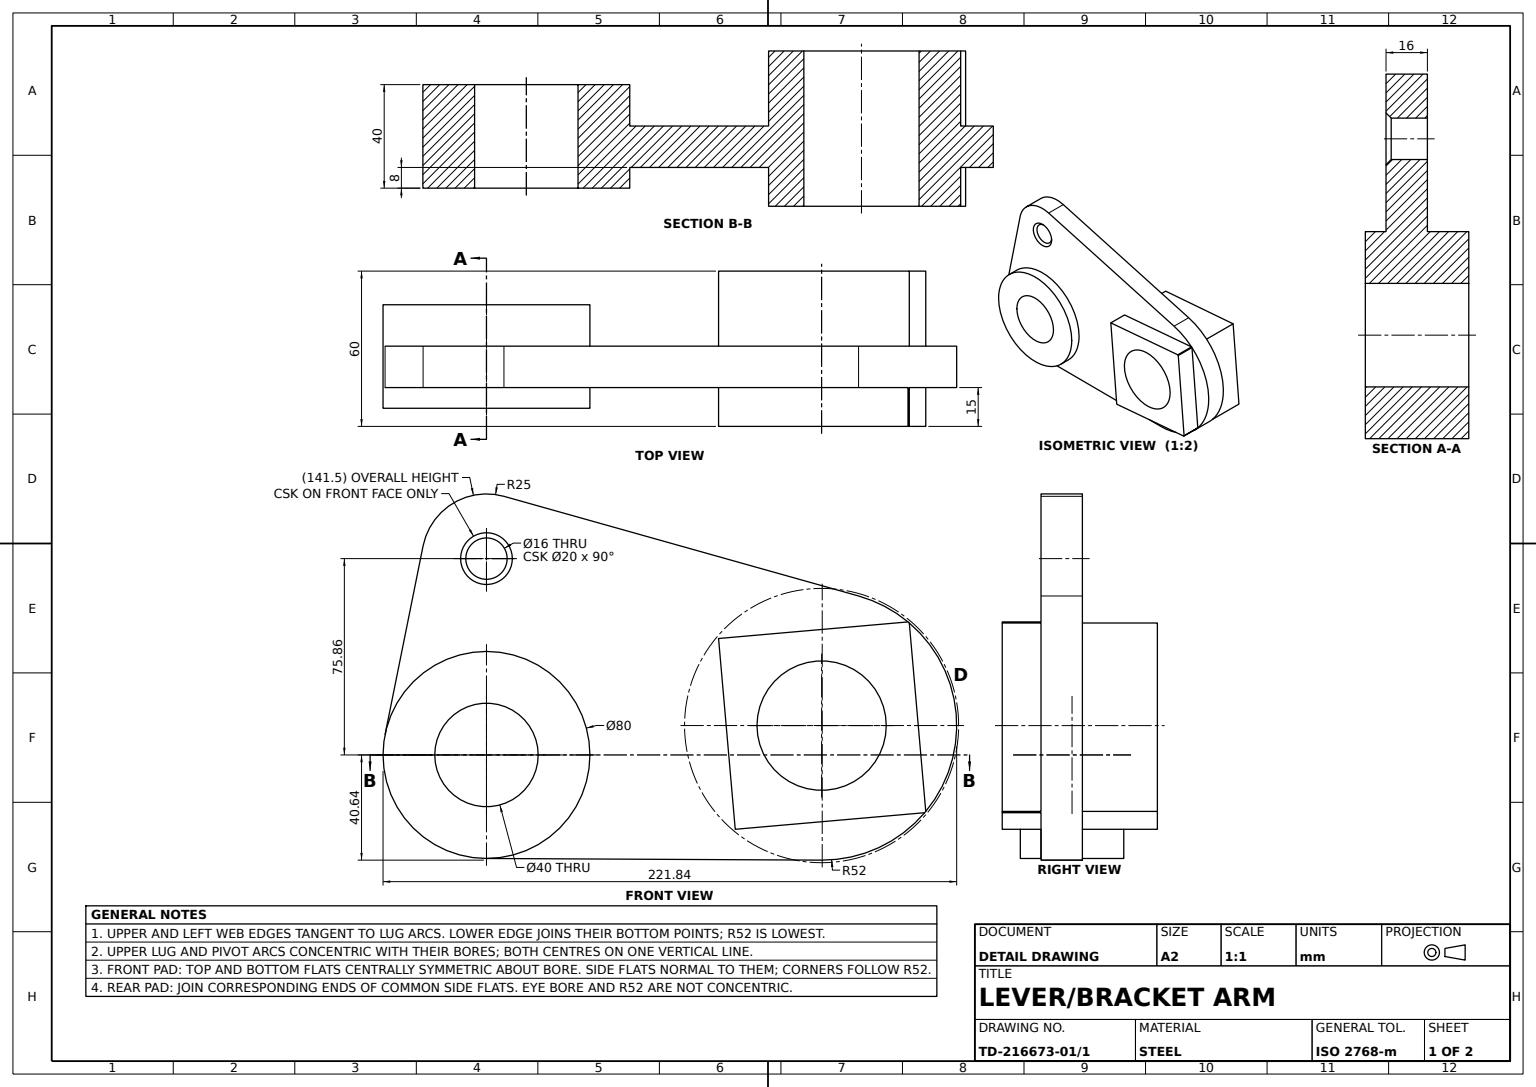
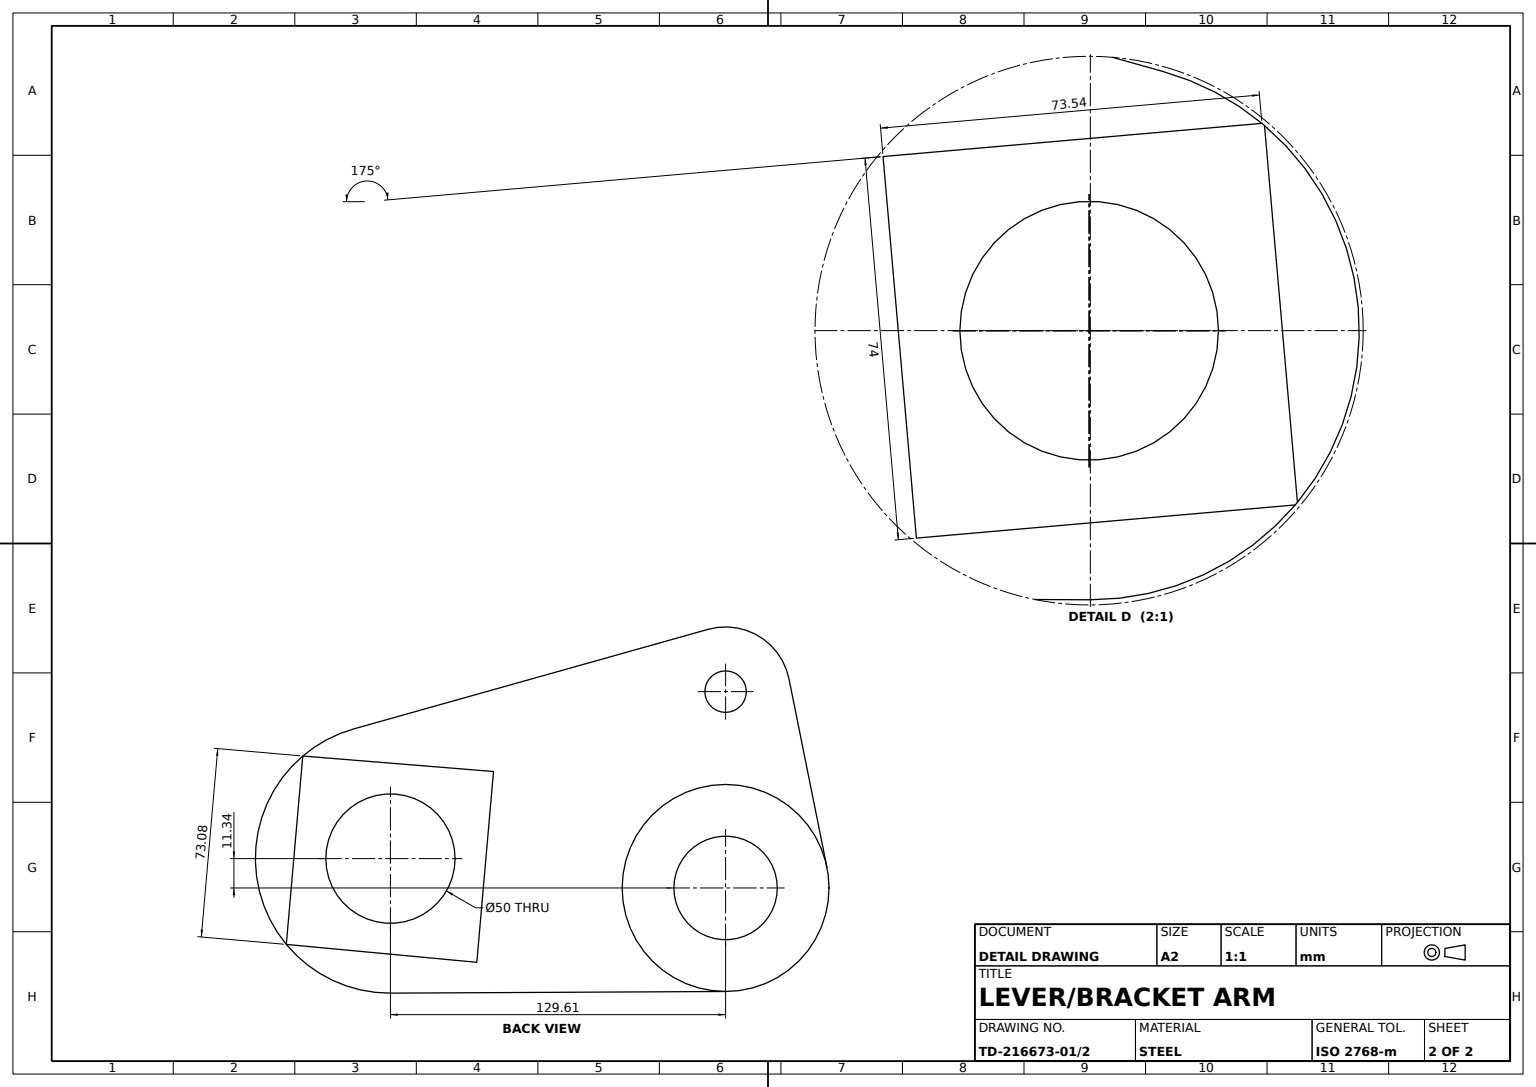
from build123d import *

# Parameters (mm, degrees)
LEVER_PLATE_DEPTH           = 16
FRONT_HUB_SKETCH_40_R       = 40
FRONT_PIVOT_HUB_40_DEPTH    = 8
REAR_START                  = 16
REAR_HUB_SKETCH_40_R        = 40
REAR_PIVOT_HUB_40_DEPTH     = 16
SMALL_HOLE_SKETCH_8_R       = 8
SMALL_HOLE_8_DEPTH          = 16
SMALL_HOLE_CHAMFER_2MM_SIZE = 2
EYE_PAD_74X74_DEPTH         = 15
EYE_BLOCK_DEPTH             = 60
EYE_BORE_SKETCH_25_R        = 25
EYE_BORE_25_DEPTH           = 60
PIVOT_BORE_SKETCH_20_R      = 20
PIVOT_BORE_20_DEPTH         = 40


with BuildPart() as part:
    # Lever Plate Profile → Lever Plate (new body)
    with BuildSketch(Plane.XY):
        with BuildLine():
            Line((143.896503384, 61.42345762), (6.758164717, 99.929217055))
            ThreePointArc((6.758164717, 99.929217055), (-13.046071322, 97.186040961), (-24.506399585, 80.803316636))
            Line((-24.506399585, 80.803316636), (-39.210239337, 7.909306617))
            ThreePointArc((-39.210239337, 7.909306617), (-30.954581767, -25.334045623), (0, -40))
            Line((0, -40), (129.839520773, -40.640513855))
            ThreePointArc((129.839520773, -40.640513855), (181.3532399, 4.26464706), (143.896503384, 61.42345762))
        make_face()
    extrude(amount=LEVER_PLATE_DEPTH)

    # Front Hub Sketch Ø40 → Front Pivot Hub Ø40 (add)
    with BuildSketch(Plane.XY.offset(16)):
        with Locations(Location((0, 0, 0), (0, 0, 168.595597299))):
            Circle(FRONT_HUB_SKETCH_40_R)
    extrude(amount=FRONT_PIVOT_HUB_40_DEPTH)

    # Rear Hub Sketch Ø40 → Rear Pivot Hub Ø40 (add)
    with BuildSketch(Plane(origin=(0, 0, 0), x_dir=(-1, 0, 0), z_dir=(0, 0, -1)).offset(REAR_START)):
        Circle(REAR_HUB_SKETCH_40_R)
    extrude(amount=-REAR_PIVOT_HUB_40_DEPTH)

    # Small Hole Sketch Ø8 → Small Hole Ø8 (cut)
    with BuildSketch(Plane.XY.offset(16)):
        with Locations((0, 75.86)):
            Circle(SMALL_HOLE_SKETCH_8_R)
    extrude(amount=-SMALL_HOLE_8_DEPTH, mode=Mode.SUBTRACT)

    # Small Hole Chamfer 2mm
    small_hole_chamfer_2mm_edges = [part.edges().sort_by_distance(p)[0] for p in [
        (-8, 75.86, 16),
    ]]
    chamfer(small_hole_chamfer_2mm_edges, length=SMALL_HOLE_CHAMFER_2MM_SIZE)

    # Eye Pad Sketch 74x74 → Eye Pad 74x74 (add)
    with BuildSketch(Plane.XY.offset(16)):
        Polygon((92.980316943, 8.134723664), (129.839520773, 11.359486145), (126.614758291, 48.218689975), (89.755554462, 44.993927493), align=None)
        Polygon((126.614758291, 48.218689975), (129.839520773, 11.359486145), (129.839520773, 48.500820134), align=None)
        with BuildLine():
            Line((129.839520773, 48.500820134), (129.839520773, 11.359486145))
            Line((129.839520773, 11.359486145), (92.980316943, 8.134723664))
            Line((92.980316943, 8.134723664), (96.205079425, -28.724480166))
            Line((96.205079425, -28.724480166), (169.462898271, -22.315251502))
            ThreePointArc((169.462898271, -22.315251502), (169.673831815, -22.065469558), (169.883190784, -21.81436639))
            Line((169.883190784, -21.81436639), (163.51425842, 50.982863644))
            ThreePointArc((163.51425842, 50.982863644), (163.264476476, 51.193797187), (163.013373308, 51.403156157))
            Line((163.013373308, 51.403156157), (129.839520773, 48.500820134))
        make_face()
    extrude(amount=EYE_PAD_74X74_DEPTH)

    # Eye Block Sketch → Eye Block (add)
    with BuildSketch(Plane.XY.offset(31)):
        Polygon((89.755554462, 44.993927493), (163.51425842, 50.982863644), (169.883190784, -21.81436639), (96.205079425, -28.724480166), align=None)
    extrude(amount=-EYE_BLOCK_DEPTH)

    # Eye Bore Sketch Ø25 → Eye Bore Ø25 (cut)
    with BuildSketch(Plane.XY.offset(31)):
        with Locations((129.609226366, 11.339337995)):
            Circle(EYE_BORE_SKETCH_25_R)
    extrude(amount=-EYE_BORE_25_DEPTH, mode=Mode.SUBTRACT)

    # Pivot Bore Sketch Ø20 → Pivot Bore Ø20 (cut)
    with BuildSketch(Plane.XY.offset(24)):
        Circle(PIVOT_BORE_SKETCH_20_R)
    extrude(amount=-PIVOT_BORE_20_DEPTH, mode=Mode.SUBTRACT)


solid = part.part
